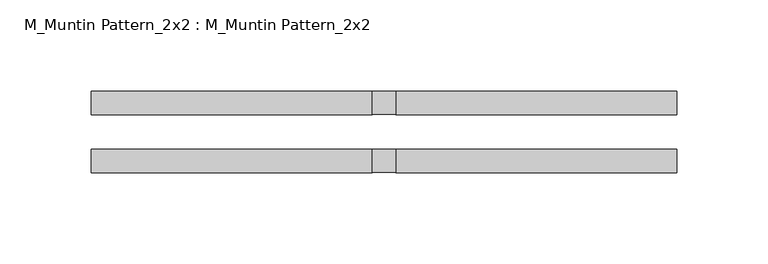
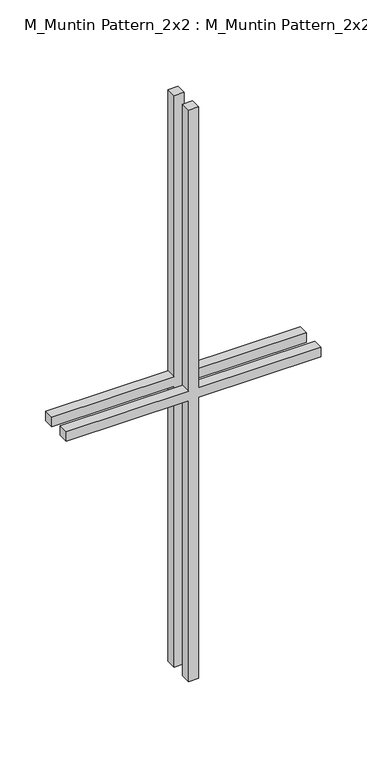
"""IFC4 building model written with IfcOpenShell, lengths in millimetres: proxy geometry, M_Muntin Pattern_2x2 : M_Muntin Pattern_2x2."""

from ifc_helpers import new_model, si_unit, frame, origin, place, context, project, spatial, polyline, outline, extrude, source, transform, mapped, element, save


def m_muntin_pattern_2x2_m_muntin_pattern_2x2_a9b7b7a9(model_context):
    return source(origin(), model_context, "Body", "SweptSolid", [
        extrude(outline(polyline([(386.5, -6.35), (386.5, -160.3375), (373.8, -160.3375), (373.8, -6.35), (0.0, -6.35), (0.0, 6.35), (373.8, 6.35), (373.8, 160.3375), (386.5, 160.3375), (386.5, 6.35), (760.3, 6.35), (760.3, -6.35), (386.5, -6.35)])), frame((0.0, -22.225, 0.0), z_axis=(0.0, 1.0, 0.0), x_axis=(0.0, 0.0, 1.0)), (0.0, 0.0, 1.0), 12.7),
        extrude(outline(polyline([(386.5, -6.35), (386.5, -160.3375), (373.8, -160.3375), (373.8, -6.35), (0.0, -6.35), (0.0, 6.35), (373.8, 6.35), (373.8, 160.3375), (386.5, 160.3375), (386.5, 6.35), (760.3, 6.35), (760.3, -6.35), (386.5, -6.35)])), frame((0.0, 9.525, 0.0), z_axis=(0.0, 1.0, 0.0), x_axis=(0.0, 0.0, 1.0)), (0.0, 0.0, 1.0), 12.7),
    ])


if __name__ == "__main__":
    model = new_model("IFC4")
    model_context = context("Model", 3, world=origin())
    ifc_project = project(units=[si_unit("LENGTHUNIT", "METRE", prefix="MILLI")], contexts=[model_context])
    site = spatial("IfcSite", under=ifc_project)
    building = spatial("IfcBuilding", under=site)
    placement = place(None, origin())
    m_muntin_pattern_2x2_m_muntin_pattern_2x2_shape = m_muntin_pattern_2x2_m_muntin_pattern_2x2_a9b7b7a9(model_context)
    element("IfcBuildingElementProxy", 1, Name="M_Muntin Pattern_2x2 : M_Muntin Pattern_2x2", ObjectType="M_Muntin Pattern_2x2 : M_Muntin Pattern_2x2", at=placement, inside=building, context=model_context, shape_type="MappedRepresentation", body=[
        mapped(m_muntin_pattern_2x2_m_muntin_pattern_2x2_shape, transform((0.0, 0.0, 0.0), x_axis=(1.0, 0.0, 0.0), y_axis=(0.0, 1.0, 0.0), z_axis=(0.0, 0.0, 1.0))),
    ])
    save(model, "model.ifc")

# Revit data of these elements
# Type "M_Muntin Pattern_2x2 : M_Muntin Pattern_2x2"
#   Width [instance default] = 3' - 11.24409"
#   Thickness = 0' - 0 1/2"
#   Height [instance default] = 3' - 11.24409"
#   Distance = 0' - 0 3/4"
#   Interior Material [instance default] = none
#   Exterior Material [instance default] = none
#   Default Elevation = 0
# Element 1 (IfcBuildingElementProxy, "M_Muntin Pattern_2x2 : M_Muntin Pattern_2x2")
#   Width = 1' - 0 5/8"
#   Height = 2' - 5.93307"
#   Interior Material = Wood - Stained
#   Exterior Material = Clad - White
#   Materials on its faces: "Clad - White", "Wood - Stained"
# Materials
#   "Clad - White": class "Wood", colour RGB 242 242 238, transparency 0, Cost = 0
#   "Wood - Stained": class "Wood", colour RGB 224 178 126, transparency 0, Cost = 0
